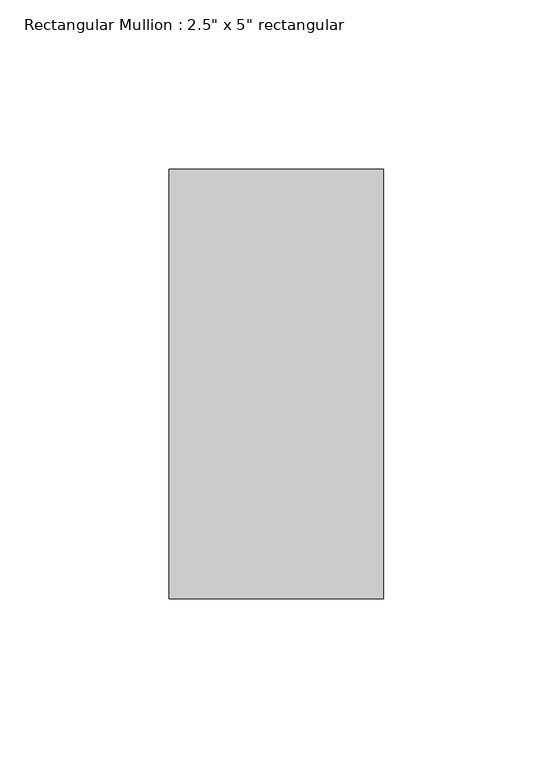
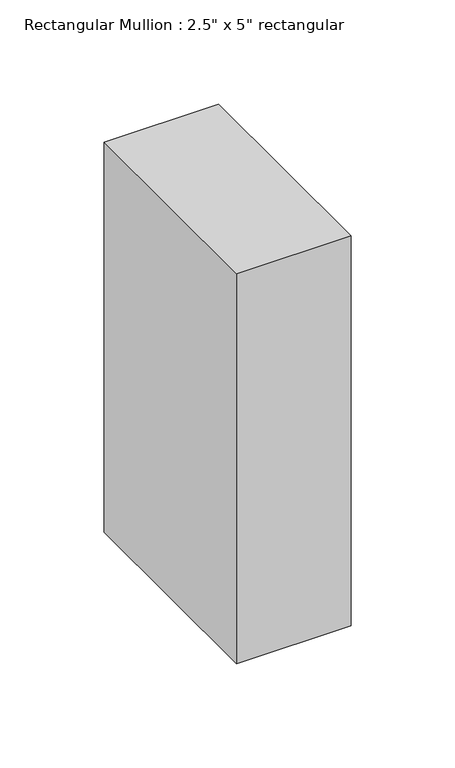
"""IFC4 building model written with IfcOpenShell, lengths in millimetres: member geometry."""

from ifc_helpers import new_model, si_unit, frame, origin, place, context, project, spatial, polyline, outline, extrude, source, transform, mapped, element, save


def member_b990fc36(model_context):
    return source(origin(), model_context, "Body", "SweptSolid", [
        extrude(outline(polyline([(31.75, 63.5), (31.75, -63.5), (-31.75, -63.5), (-31.75, 63.5), (31.75, 63.5)])), frame((0.0, 0.0, -228.6), z_axis=(0.0, 0.0, 1.0), x_axis=(1.0, 0.0, 0.0)), (0.0, 0.0, 1.0), 228.6),
    ])


if __name__ == "__main__":
    model = new_model("IFC4")
    model_context = context("Model", 3, world=origin())
    ifc_project = project(units=[si_unit("LENGTHUNIT", "METRE", prefix="MILLI")], contexts=[model_context])
    site = spatial("IfcSite", under=ifc_project)
    building = spatial("IfcBuilding", under=site)
    placement = place(None, origin())
    member_shape = member_b990fc36(model_context)
    element("IfcMember", 1, ObjectType="Rectangular Mullion : 2.5\" x 5\" rectangular", at=placement, inside=building, context=model_context, shape_type="MappedRepresentation", body=[
        mapped(member_shape, transform((0.0, 0.0, 0.0), x_axis=(1.0, 0.0, 0.0), y_axis=(0.0, 1.0, 0.0), z_axis=(0.0, 0.0, 1.0))),
    ])
    save(model, "model.ifc")

# Revit data of these elements
# Type "Rectangular Mullion : 2.5\" x 5\" rectangular"
#   built-in parameter 1007304 = 0.416667 (stored number, unit not read)
#   built-in parameter 1007301 = 0.104167 (stored number, unit not read)
#   built-in parameter 1007300 = 0.104167 (stored number, unit not read)
# Element 1 (IfcMember, "Rectangular Mullion : 2.5\" x 5\" rectangular")
#   Materials on its faces: "Aluminum"
# Materials
#   "Aluminum": class "Metal", colour RGB 247 247 247, transparency 0, Description = "Aluminum 6061", Cost = 0
